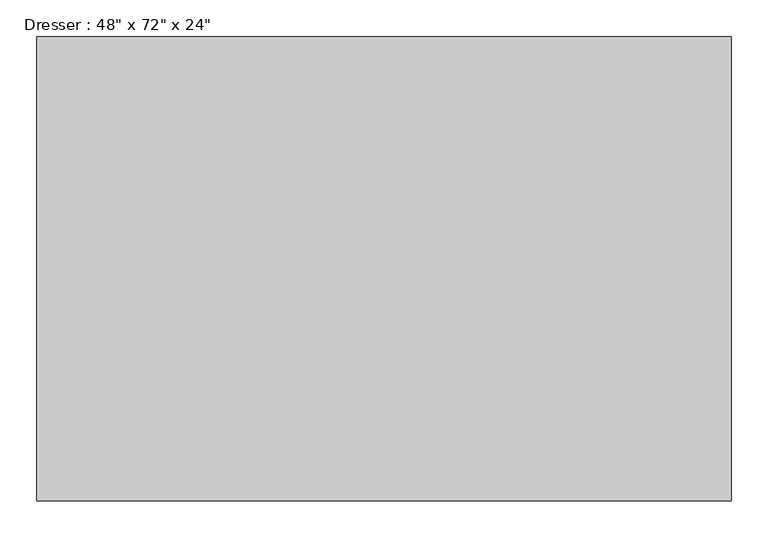
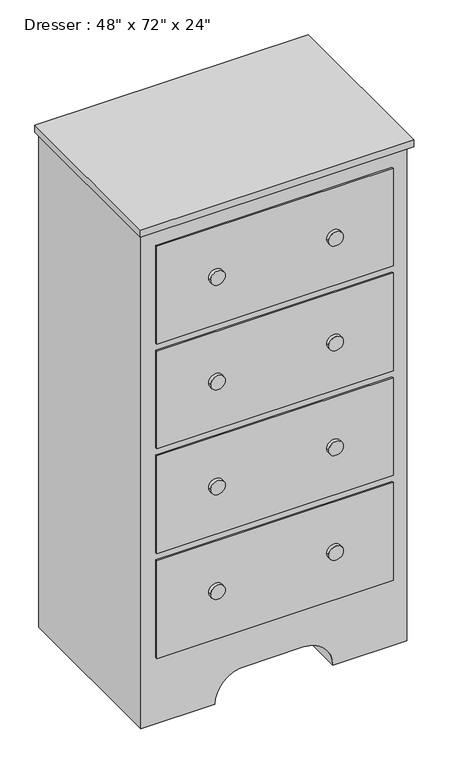
"""IFC4 building model written with IfcOpenShell, lengths in millimetres: furniture geometry."""

from ifc_helpers import new_model, si_unit, point, frame, frame_2d, origin, place, context, project, spatial, polyline, circle_curve, trimmed, segment, composite_curve, outline, extrude, source, transform, mapped, element, save


def furniture_33655958(model_context):
    return source(origin(), model_context, "Body", "SweptSolid", [
        extrude(outline(polyline([(200.7067402, -58.3629541), (200.7067402, -687.0129541), (-739.0932598, -687.0129541), (-739.0932598, -58.3629541), (200.7067402, -58.3629541)])), frame((0.0, 0.0, 1803.4), z_axis=(0.0, 0.0, 1.0), x_axis=(1.0, 0.0, 0.0)), (0.0, 0.0, 1.0), 25.4),
        extrude(outline(composite_curve([segment(polyline([(0.0, 188.0067402), (1803.4, 188.0067402), (1803.4, -726.3932598), (0.0, -726.3932598), (0.0, -472.3932598)]), True, "CONTINUOUS"), segment(trimmed(circle_curve(frame_2d((0.0, -370.7932598)), 101.6), [point((0.0, -472.3932598))], [point((101.6, -370.7932598))], True, "CARTESIAN"), True, "CONTINUOUS"), segment(polyline([(101.6, -370.7932598), (101.6, -167.5932598)]), True, "CONTINUOUS"), segment(trimmed(circle_curve(frame_2d((0.0, -167.5932598)), 101.6), [point((101.6, -167.5932598))], [point((0.0, -65.9932598))], True, "CARTESIAN"), True, "CONTINUOUS"), segment(polyline([(0.0, -65.9932598), (0.0, 188.0067402)]), True, "CONTINUOUS")], self_intersect=False)), frame((0.0, -667.9629541, 0.0), z_axis=(0.0, 1.0, 0.0), x_axis=(0.0, 0.0, 1.0)), (0.0, 0.0, 1.0), 609.6),
        extrude(outline(composite_curve([segment(trimmed(circle_curve(frame_2d((1562.1, -65.9932598)), 25.4), [point((1562.1, -91.3932598))], [point((1562.1, -40.5932598))], False, "CARTESIAN"), True, "CONTINUOUS"), segment(trimmed(circle_curve(frame_2d((1562.1, -65.9932598)), 25.4), [point((1562.1, -40.5932598))], [point((1562.1, -91.3932598))], False, "CARTESIAN"), True, "CONTINUOUS")], self_intersect=False)), frame((0.0, -687.0129541, 0.0), z_axis=(0.0, 1.0, 0.0), x_axis=(0.0, 0.0, 1.0)), (0.0, 0.0, 1.0), 12.7),
        extrude(outline(composite_curve([segment(trimmed(circle_curve(frame_2d((1181.1, -65.9932598)), 25.4), [point((1181.1, -91.3932598))], [point((1181.1, -40.5932598))], False, "CARTESIAN"), True, "CONTINUOUS"), segment(trimmed(circle_curve(frame_2d((1181.1, -65.9932598)), 25.4), [point((1181.1, -40.5932598))], [point((1181.1, -91.3932598))], False, "CARTESIAN"), True, "CONTINUOUS")], self_intersect=False)), frame((0.0, -687.0129541, 0.0), z_axis=(0.0, 1.0, 0.0), x_axis=(0.0, 0.0, 1.0)), (0.0, 0.0, 1.0), 12.7),
        extrude(outline(composite_curve([segment(trimmed(circle_curve(frame_2d((800.1, -65.9932598)), 25.4), [point((800.1, -91.3932598))], [point((800.1, -40.5932598))], False, "CARTESIAN"), True, "CONTINUOUS"), segment(trimmed(circle_curve(frame_2d((800.1, -65.9932598)), 25.4), [point((800.1, -40.5932598))], [point((800.1, -91.3932598))], False, "CARTESIAN"), True, "CONTINUOUS")], self_intersect=False)), frame((0.0, -687.0129541, 0.0), z_axis=(0.0, 1.0, 0.0), x_axis=(0.0, 0.0, 1.0)), (0.0, 0.0, 1.0), 12.7),
        extrude(outline(composite_curve([segment(trimmed(circle_curve(frame_2d((419.1, -65.9932598)), 25.4), [point((419.1, -91.3932598))], [point((419.1, -40.5932598))], False, "CARTESIAN"), True, "CONTINUOUS"), segment(trimmed(circle_curve(frame_2d((419.1, -65.9932598)), 25.4), [point((419.1, -40.5932598))], [point((419.1, -91.3932598))], False, "CARTESIAN"), True, "CONTINUOUS")], self_intersect=False)), frame((0.0, -687.0129541, 0.0), z_axis=(0.0, 1.0, 0.0), x_axis=(0.0, 0.0, 1.0)), (0.0, 0.0, 1.0), 12.7),
        extrude(outline(composite_curve([segment(trimmed(circle_curve(frame_2d((419.1, -472.3932598)), 25.4), [point((419.1, -497.7932598))], [point((419.1, -446.9932598))], False, "CARTESIAN"), True, "CONTINUOUS"), segment(trimmed(circle_curve(frame_2d((419.1, -472.3932598)), 25.4), [point((419.1, -446.9932598))], [point((419.1, -497.7932598))], False, "CARTESIAN"), True, "CONTINUOUS")], self_intersect=False)), frame((0.0, -687.0129541, 0.0), z_axis=(0.0, 1.0, 0.0), x_axis=(0.0, 0.0, 1.0)), (0.0, 0.0, 1.0), 12.7),
        extrude(outline(composite_curve([segment(trimmed(circle_curve(frame_2d((800.1, -472.3932598)), 25.4), [point((800.1, -497.7932598))], [point((800.1, -446.9932598))], False, "CARTESIAN"), True, "CONTINUOUS"), segment(trimmed(circle_curve(frame_2d((800.1, -472.3932598)), 25.4), [point((800.1, -446.9932598))], [point((800.1, -497.7932598))], False, "CARTESIAN"), True, "CONTINUOUS")], self_intersect=False)), frame((0.0, -687.0129541, 0.0), z_axis=(0.0, 1.0, 0.0), x_axis=(0.0, 0.0, 1.0)), (0.0, 0.0, 1.0), 12.7),
        extrude(outline(composite_curve([segment(trimmed(circle_curve(frame_2d((1181.1, -472.3932598)), 25.4), [point((1181.1, -497.7932598))], [point((1181.1, -446.9932598))], False, "CARTESIAN"), True, "CONTINUOUS"), segment(trimmed(circle_curve(frame_2d((1181.1, -472.3932598)), 25.4), [point((1181.1, -446.9932598))], [point((1181.1, -497.7932598))], False, "CARTESIAN"), True, "CONTINUOUS")], self_intersect=False)), frame((0.0, -687.0129541, 0.0), z_axis=(0.0, 1.0, 0.0), x_axis=(0.0, 0.0, 1.0)), (0.0, 0.0, 1.0), 12.7),
        extrude(outline(composite_curve([segment(trimmed(circle_curve(frame_2d((1562.1, -472.3932598)), 25.4), [point((1562.1, -497.7932598))], [point((1562.1, -446.9932598))], False, "CARTESIAN"), True, "CONTINUOUS"), segment(trimmed(circle_curve(frame_2d((1562.1, -472.3932598)), 25.4), [point((1562.1, -446.9932598))], [point((1562.1, -497.7932598))], False, "CARTESIAN"), True, "CONTINUOUS")], self_intersect=False)), frame((0.0, -687.0129541, 0.0), z_axis=(0.0, 1.0, 0.0), x_axis=(0.0, 0.0, 1.0)), (0.0, 0.0, 1.0), 12.7),
        extrude(outline(polyline([(137.2067402, -674.3129541), (-675.5932598, -674.3129541), (-675.5932598, -667.9629541), (137.2067402, -667.9629541), (137.2067402, -674.3129541)])), frame((0.0, 0.0, 1384.3), z_axis=(0.0, 0.0, 1.0), x_axis=(1.0, 0.0, 0.0)), (0.0, 0.0, 1.0), 355.6),
        extrude(outline(polyline([(137.2067402, -674.3129541), (-675.5932598, -674.3129541), (-675.5932598, -667.9629541), (137.2067402, -667.9629541), (137.2067402, -674.3129541)])), frame((0.0, 0.0, 1003.3), z_axis=(0.0, 0.0, 1.0), x_axis=(1.0, 0.0, 0.0)), (0.0, 0.0, 1.0), 355.6),
        extrude(outline(polyline([(137.2067402, -674.3129541), (-675.5932598, -674.3129541), (-675.5932598, -667.9629541), (137.2067402, -667.9629541), (137.2067402, -674.3129541)])), frame((0.0, 0.0, 622.3), z_axis=(0.0, 0.0, 1.0), x_axis=(1.0, 0.0, 0.0)), (0.0, 0.0, 1.0), 355.6),
        extrude(outline(polyline([(137.2067402, -674.3129541), (-675.5932598, -674.3129541), (-675.5932598, -667.9629541), (137.2067402, -667.9629541), (137.2067402, -674.3129541)])), frame((0.0, 0.0, 241.3), z_axis=(0.0, 0.0, 1.0), x_axis=(1.0, 0.0, 0.0)), (0.0, 0.0, 1.0), 355.6),
    ])


if __name__ == "__main__":
    model = new_model("IFC4")
    model_context = context("Model", 3, world=origin())
    ifc_project = project(units=[si_unit("LENGTHUNIT", "METRE", prefix="MILLI")], contexts=[model_context])
    site = spatial("IfcSite", under=ifc_project)
    building = spatial("IfcBuilding", under=site)
    placement = place(None, origin())
    furniture_shape = furniture_33655958(model_context)
    element("IfcFurniture", 1, ObjectType="Dresser : 48\" x 72\" x 24\"", at=placement, inside=building, context=model_context, shape_type="MappedRepresentation", body=[
        mapped(furniture_shape, transform((0.0, 0.0, 0.0), x_axis=(1.0, 0.0, 0.0), y_axis=(0.0, 1.0, 0.0), z_axis=(0.0, 0.0, 1.0))),
    ])
    save(model, "model.ifc")

# Revit data of these elements
# Type "Dresser : 48\" x 72\" x 24\""
#   Assembly Code = "E2020200"
#   Depth = 2' - 0"
#   Height = 6' - 0"
#   Width = 3' - 0"
#   Dresser Material = Wood - Teak
#   Drawer Material = Wood - Teak
#   Knob Material = Cherry
#   Default Elevation = 0
# Element 1 (IfcFurniture, "Dresser : 48\" x 72\" x 24\"")
#   Materials on its faces: "Laminate, Ivory, Matte", "Cherry", "Wood - Teak"
# Materials
#   "Wood - Teak": class "Wood", colour RGB 145 112 90, transparency 0
#   "Cherry": class "Wood", colour RGB 226 177 128, transparency 0, Description = "Prunus Serotina", Cost = 0
#   "Laminate, Ivory, Matte": class "Plastic", colour RGB 247 247 239, transparency 0, Description = "Plastic Laminate - Ivory, Matte", Cost = 0
